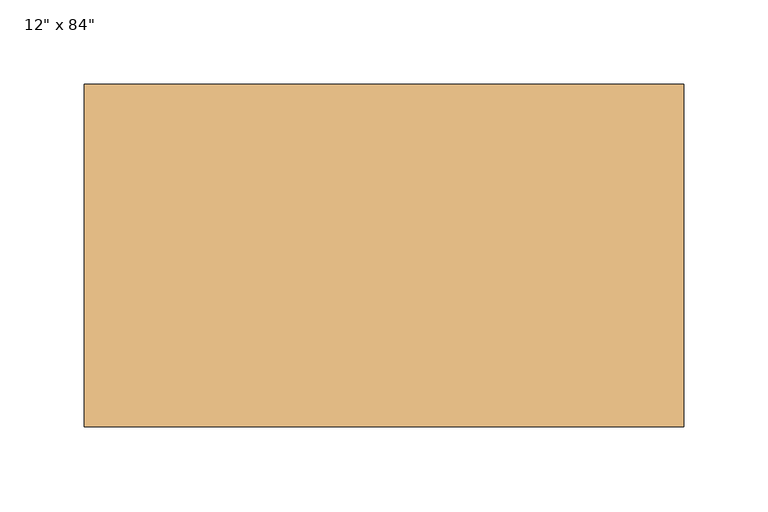
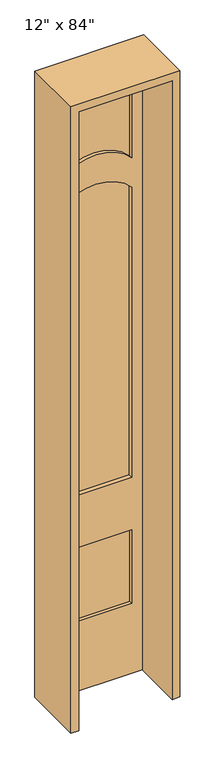
"""IFC4 building model written with IfcOpenShell, lengths in millimetres: door geometry."""

from ifc_helpers import new_model, si_unit, point, frame, frame_2d, origin, place, context, project, spatial, polyline, circle_curve, trimmed, segment, composite_curve, outline, extrude, source, transform, mapped, element, save


def door_c3736dc5(model_context):
    return source(origin(), model_context, "Body", "SweptSolid", [
        extrude(outline(polyline([(117.475, 75.1416667), (-117.475, 75.1416667), (-117.475, 86.7833333), (117.475, 86.7833333), (117.475, 75.1416667)])), frame((0.0, 0.0, 241.3), z_axis=(0.0, 0.0, 1.0), x_axis=(1.0, 0.0, 0.0)), (0.0, 0.0, 1.0), 254.0),
        extrude(outline(composite_curve([segment(polyline([(1778.0, 117.475), (2012.95, 117.475), (2012.95, -117.475), (1778.0, -117.475)]), True, "CONTINUOUS"), segment(trimmed(circle_curve(frame_2d((1667.5695312, 0.0)), 161.2304687), [point((1778.0, -117.475))], [point((1778.0, 117.475))], True, "CARTESIAN"), True, "CONTINUOUS")], self_intersect=False)), frame((0.0, 75.1416667, 0.0), z_axis=(0.0, 1.0, 0.0), x_axis=(0.0, 0.0, 1.0)), (0.0, 0.0, 1.0), 11.6416667),
        extrude(outline(polyline([(2133.6, -152.4), (0.0, -152.4), (0.0, 152.4), (2133.6, 152.4), (2133.6, -152.4)]), holes=[composite_curve([segment(polyline([(676.275, -117.475), (1676.4, -117.475)]), True, "CONTINUOUS"), segment(trimmed(circle_curve(frame_2d((1565.9695312, 0.0)), 161.2304688), [point((1676.4, -117.475))], [point((1676.4, 117.475))], True, "CARTESIAN"), True, "CONTINUOUS"), segment(polyline([(1676.4, 117.475), (676.275, 117.475), (676.275, -117.475)]), True, "CONTINUOUS")], self_intersect=False), polyline([(495.3, -117.475), (495.3, 117.475), (241.3, 117.475), (241.3, -117.475), (495.3, -117.475)]), composite_curve([segment(polyline([(2012.95, -117.475), (2012.95, 117.475), (1778.0, 117.475)]), True, "CONTINUOUS"), segment(trimmed(circle_curve(frame_2d((1667.5695312, 0.0)), 161.2304687), [point((1778.0, 117.475))], [point((1778.0, -117.475))], False, "CARTESIAN"), True, "CONTINUOUS"), segment(polyline([(1778.0, -117.475), (2012.95, -117.475)]), True, "CONTINUOUS")], self_intersect=False)]), frame((0.0, 63.5, 0.0), z_axis=(0.0, 1.0, 0.0), x_axis=(0.0, 0.0, 1.0)), (0.0, 0.0, 1.0), 34.925),
        extrude(outline(polyline([(0.0, 152.4), (0.0, 177.8), (2159.0, 177.8), (2159.0, -177.8), (0.0, -177.8), (0.0, -152.4), (2133.6, -152.4), (2133.6, 152.4), (0.0, 152.4)])), frame((0.0, -104.775, 0.0), z_axis=(0.0, 1.0, 0.0), x_axis=(0.0, 0.0, 1.0)), (0.0, 0.0, 1.0), 203.2),
        extrude(outline(composite_curve([segment(polyline([(676.275, -117.475), (676.275, 117.475), (1676.4, 117.475)]), True, "CONTINUOUS"), segment(trimmed(circle_curve(frame_2d((1565.9695312, 0.0)), 161.2304688), [point((1676.4, 117.475))], [point((1676.4, -117.475))], False, "CARTESIAN"), True, "CONTINUOUS"), segment(polyline([(1676.4, -117.475), (676.275, -117.475)]), True, "CONTINUOUS")], self_intersect=False)), frame((0.0, 77.47, 0.0), z_axis=(0.0, 1.0, 0.0), x_axis=(0.0, 0.0, 1.0)), (0.0, 0.0, 1.0), 6.985),
    ])


if __name__ == "__main__":
    model = new_model("IFC4")
    model_context = context("Model", 3, world=origin())
    ifc_project = project(units=[si_unit("LENGTHUNIT", "METRE", prefix="MILLI")], contexts=[model_context])
    site = spatial("IfcSite", under=ifc_project)
    building = spatial("IfcBuilding", under=site)
    placement = place(None, origin())
    door_shape = door_c3736dc5(model_context)
    element("IfcDoor", 1, ObjectType="12\" x 84\"", at=placement, inside=building, context=model_context, shape_type="MappedRepresentation", body=[
        mapped(door_shape, transform((0.0, 0.0, 0.0), x_axis=(1.0, 0.0, 0.0), y_axis=(0.0, 1.0, 0.0), z_axis=(0.0, 0.0, 1.0))),
    ])
    save(model, "model.ifc")

# Revit data of these elements
# Type "12\" x 84\""
#   Type Mark = "10"
#   Assembly Code = "B2030100"
#   Analytic Construction = "French door, wood frame with single glass"
#   Radius = 0' - 6 89/256"
#   Lock Rail = 0' - 7 1/8"
#   Thickness = 0' - 1 3/8"
#   Thermal Resistance (R) = 1.0696 (h·ft²·°F)/BTU
#   Stiles = 0' - 1 3/8"
#   Rough Width = 1' - 2"
#   Rough Height = 7' - 1"
#   Height = 7' - 0"
#   Width = 1' - 0"
#   Heat Transfer Coefficient (U) = 0.9350 BTU/(h·ft²·°F)
#   Door Offset [instance default] = 0' - 0"
#   Bottom Rail = 0' - 9 1/2"
#   Function = 1
#   Trim Material = Cherry
#   Panel Material = Cherry
#   Glazing = Glass
#   Frame Material = Cherry
#   Visual Light Transmittance = 0
#   Solar Heat Gain Coefficient = 0
#   Wall Closure = (empty or 0)
#   Construction Type = (empty or 0)
# Element 1 (IfcDoor, "12\" x 84\"")
#   Materials on its faces: "Cherry", "Glass"
# Materials
#   "Cherry": class "Wood", colour RGB 226 177 128, transparency 0, Description = "Prunus Serotina", Cost = 0
#   "Glass": class "Glass", colour RGB 0 128 192, transparency 0.75, Description = "Soda Lime Glass", Cost = 0
